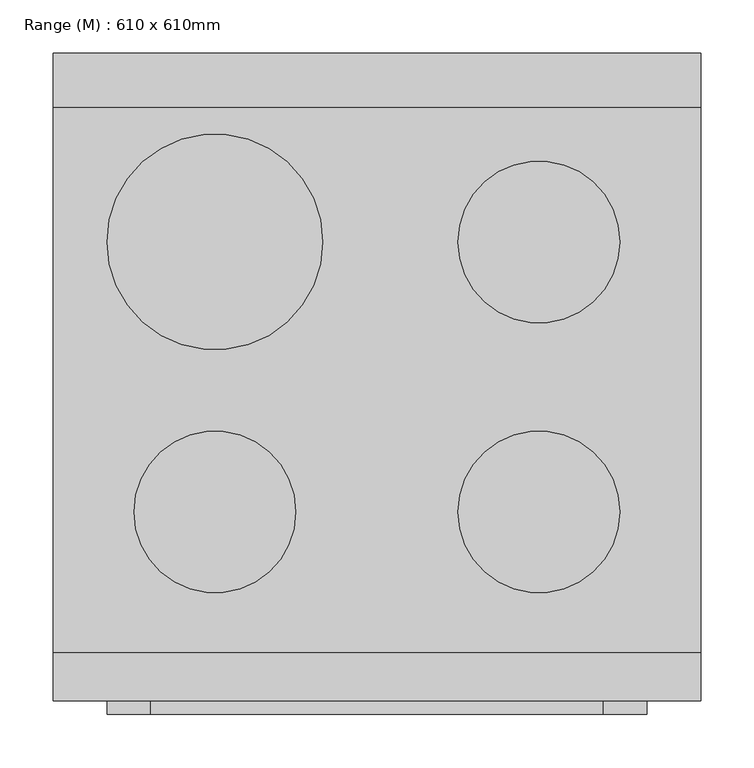
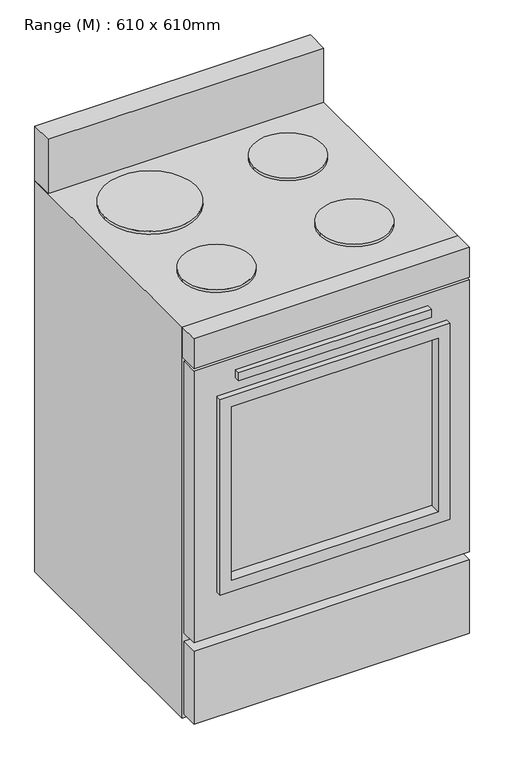
"""IFC4 building model written with IfcOpenShell, lengths in millimetres: proxy geometry, Range (M) : 610 x 610mm."""

from ifc_helpers import new_model, si_unit, point, frame, frame_2d, origin, place, context, project, spatial, polyline, circle_curve, trimmed, segment, composite_curve, outline, extrude, source, transform, mapped, element, save


def range_m_610_x_610mm_88bdc8d1(model_context):
    return source(origin(), model_context, "Body", "SweptSolid", [
        extrude(outline(polyline([(517.925, -12.7), (91.687309, -12.7), (91.687309, 0.0), (517.925, 0.0), (517.925, -12.7)])), frame((0.0, 0.0, 791.2768639), z_axis=(0.0, 0.0, 1.0), x_axis=(1.0, 0.0, 0.0)), (0.0, 0.0, 1.0), 19.05),
        extrude(outline(polyline([(533.8, 12.7), (76.2, 12.7), (76.2, 19.05), (533.8, 19.05), (533.8, 12.7)])), frame((0.0, 0.0, 330.2), z_axis=(0.0, 0.0, 1.0), x_axis=(1.0, 0.0, 0.0)), (0.0, 0.0, 1.0), 406.4),
        extrude(outline(polyline([(610.0, 0.0), (0.0, 0.0), (0.0, 45.0), (610.0, 45.0), (610.0, 0.0)])), frame((0.0, 0.0, 844.7720355), z_axis=(0.0, 0.0, 1.0), x_axis=(1.0, 0.0, 0.0)), (0.0, 0.0, 1.0), 69.6279645),
        extrude(outline(polyline([(762.0, 559.2), (762.0, 50.8), (304.8, 50.8), (304.8, 559.2), (762.0, 559.2)]), holes=[polyline([(736.6, 533.8), (330.2, 533.8), (330.2, 76.2), (736.6, 76.2), (736.6, 533.8)])]), frame((0.0, -12.7, 0.0), z_axis=(0.0, 1.0, 0.0), x_axis=(0.0, 0.0, 1.0)), (0.0, 0.0, 1.0), 38.1),
        extrude(outline(composite_curve([segment(trimmed(circle_curve(frame_2d((152.4, 432.2)), 101.6), [point((50.8, 432.2))], [point((254.0, 432.2))], False, "CARTESIAN"), True, "CONTINUOUS"), segment(trimmed(circle_curve(frame_2d((152.4, 432.2)), 101.6), [point((254.0, 432.2))], [point((50.8, 432.2))], False, "CARTESIAN"), True, "CONTINUOUS")], self_intersect=False)), frame((0.0, 0.0, 914.4), z_axis=(0.0, 0.0, 1.0), x_axis=(1.0, 0.0, 0.0)), (0.0, 0.0, 1.0), 6.35),
        extrude(outline(composite_curve([segment(trimmed(circle_curve(frame_2d((457.6, 432.2)), 76.2), [point((381.4, 432.2))], [point((533.8, 432.2))], False, "CARTESIAN"), True, "CONTINUOUS"), segment(trimmed(circle_curve(frame_2d((457.6, 432.2)), 76.2), [point((533.8, 432.2))], [point((381.4, 432.2))], False, "CARTESIAN"), True, "CONTINUOUS")], self_intersect=False)), frame((0.0, 0.0, 914.4), z_axis=(0.0, 0.0, 1.0), x_axis=(1.0, 0.0, 0.0)), (0.0, 0.0, 1.0), 6.35),
        extrude(outline(composite_curve([segment(trimmed(circle_curve(frame_2d((457.6, 177.8)), 76.2), [point((381.4, 177.8))], [point((533.8, 177.8))], False, "CARTESIAN"), True, "CONTINUOUS"), segment(trimmed(circle_curve(frame_2d((457.6, 177.8)), 76.2), [point((533.8, 177.8))], [point((381.4, 177.8))], False, "CARTESIAN"), True, "CONTINUOUS")], self_intersect=False)), frame((0.0, 0.0, 914.4), z_axis=(0.0, 0.0, 1.0), x_axis=(1.0, 0.0, 0.0)), (0.0, 0.0, 1.0), 6.35),
        extrude(outline(composite_curve([segment(trimmed(circle_curve(frame_2d((152.4, 177.8)), 76.2), [point((76.2, 177.8))], [point((228.6, 177.8))], False, "CARTESIAN"), True, "CONTINUOUS"), segment(trimmed(circle_curve(frame_2d((152.4, 177.8)), 76.2), [point((228.6, 177.8))], [point((76.2, 177.8))], False, "CARTESIAN"), True, "CONTINUOUS")], self_intersect=False)), frame((0.0, 0.0, 914.4), z_axis=(0.0, 0.0, 1.0), x_axis=(1.0, 0.0, 0.0)), (0.0, 0.0, 1.0), 6.35),
        extrude(outline(polyline([(25.4, 610.0), (584.6, 610.0), (584.6, 584.6), (25.4, 584.6), (25.4, 610.0)])), frame((0.0, 0.0, 254.0), z_axis=(0.0, 0.0, 1.0), x_axis=(1.0, 0.0, 0.0)), (0.0, 0.0, 1.0), 635.2220355),
        extrude(outline(polyline([(838.4220355, 610.0), (838.4220355, 0.0), (203.2, 0.0), (203.2, 610.0), (838.4220355, 610.0)]), holes=[polyline([(762.0, 559.2), (304.8, 559.2), (304.8, 50.8), (762.0, 50.8), (762.0, 559.2)])]), frame((0.0, 0.0, 0.0), z_axis=(0.0, 1.0, 0.0), x_axis=(0.0, 0.0, 1.0)), (0.0, 0.0, 1.0), 38.1),
        extrude(outline(polyline([(610.0, 0.0), (0.0, 0.0), (0.0, 38.1), (610.0, 38.1), (610.0, 0.0)])), frame((0.0, 0.0, 12.7), z_axis=(0.0, 0.0, 1.0), x_axis=(1.0, 0.0, 0.0)), (0.0, 0.0, 1.0), 171.45),
        extrude(outline(polyline([(914.4, 610.0), (914.4, 0.0), (0.0, 0.0), (0.0, 610.0), (914.4, 610.0)]), holes=[polyline([(889.2220355, 584.6), (254.0, 584.6), (254.0, 25.4), (889.2220355, 25.4), (889.2220355, 584.6)])]), frame((0.0, 45.0, 0.0), z_axis=(0.0, 1.0, 0.0), x_axis=(0.0, 0.0, 1.0)), (0.0, 0.0, 1.0), 565.0),
        extrude(outline(polyline([(610.0, 610.0), (610.0, 559.2), (0.0, 559.2), (0.0, 610.0), (610.0, 610.0)])), frame((0.0, 0.0, 914.4), z_axis=(0.0, 0.0, 1.0), x_axis=(1.0, 0.0, 0.0)), (0.0, 0.0, 1.0), 127.0),
    ])


if __name__ == "__main__":
    model = new_model("IFC4")
    model_context = context("Model", 3, world=origin())
    ifc_project = project(units=[si_unit("LENGTHUNIT", "METRE", prefix="MILLI")], contexts=[model_context])
    site = spatial("IfcSite", under=ifc_project)
    building = spatial("IfcBuilding", under=site)
    placement = place(None, origin())
    range_m_610_x_610mm_shape = range_m_610_x_610mm_88bdc8d1(model_context)
    element("IfcBuildingElementProxy", 1, Name="Range (M) : 610 x 610mm", ObjectType="Range (M) : 610 x 610mm", at=placement, inside=building, context=model_context, shape_type="MappedRepresentation", body=[
        mapped(range_m_610_x_610mm_shape, transform((0.0, 0.0, 0.0), x_axis=(1.0, 0.0, 0.0), y_axis=(0.0, 1.0, 0.0), z_axis=(0.0, 0.0, 1.0))),
    ])
    save(model, "model.ifc")

# Revit data of these elements
# Type "Range (M) : 610 x 610mm"
#   Depth = 2' - 0.01575"
#   Width = 2' - 0.01575"
#   Burner Material = Metal - Chrome
#   Range Material = Metal - Painted Finish - Ivory,Matte
#   Default Elevation = 0
#   Assembly Code = ""
# Element 1 (IfcBuildingElementProxy, "Range (M) : 610 x 610mm")
#   Materials on its faces: "Metal - Painted Finish - Ivory,Matte", "Metal - Chrome", "Glass"
# Materials
#   "Metal - Chrome": class "Metal", colour RGB 17 17 17, transparency 0
#   "Metal - Painted Finish - Ivory,Matte": colour RGB 247 247 239, transparency 0
#   "Glass": class "Glass", colour RGB 0 128 192, transparency 0.75, Description = "Soda Lime Glass", Cost = 0
